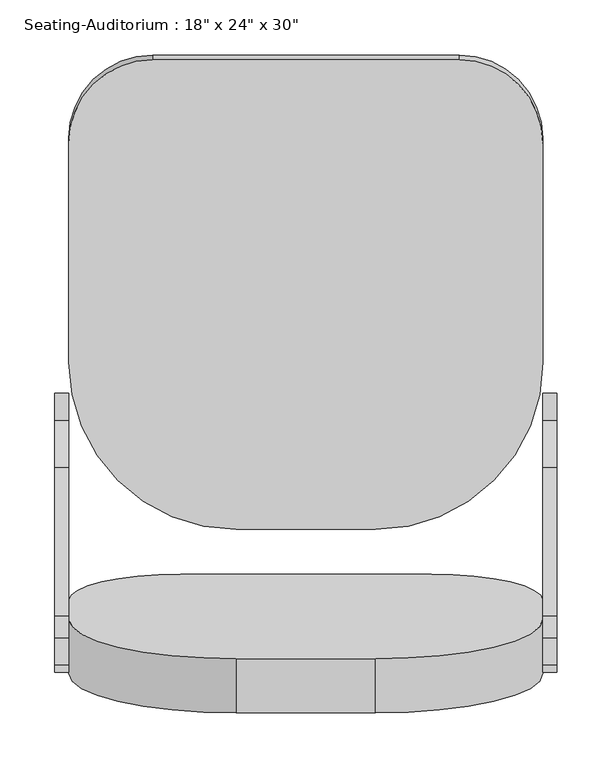
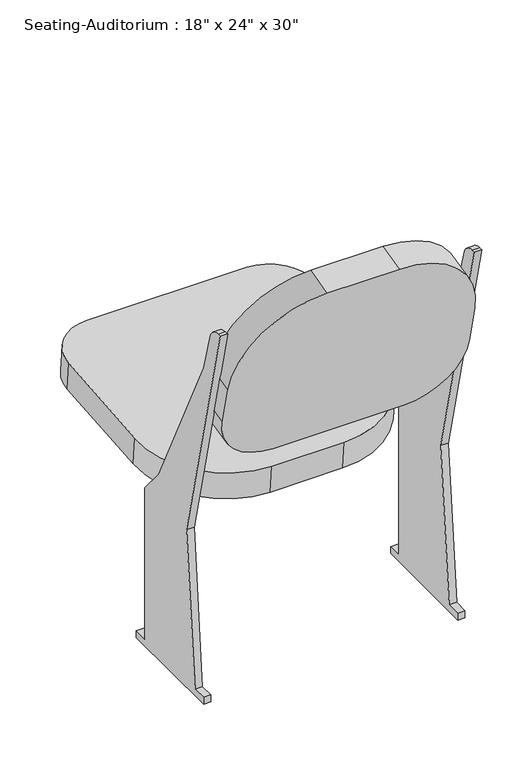
"""IFC4 building model written with IfcOpenShell, lengths in millimetres: furniture geometry."""

from ifc_helpers import new_model, si_unit, point, frame, frame_2d, origin, place, context, project, spatial, polyline, circle_curve, trimmed, segment, composite_curve, outline, extrude, source, transform, mapped, element, save


def furniture_3d1d9cbc(model_context):
    return source(origin(), model_context, "Body", "SweptSolid", [
        extrude(outline(composite_curve([segment(polyline([(0.0, 0.0), (127.0, 0.0)]), True, "CONTINUOUS"), segment(trimmed(circle_curve(frame_2d((127.0, -152.4)), 152.4), [point((127.0, 0.0))], [point((279.4, -152.4))], False, "CARTESIAN"), True, "CONTINUOUS"), segment(polyline([(279.4, -152.4), (279.4, -224.0588601)]), True, "CONTINUOUS"), segment(trimmed(circle_curve(frame_2d((177.8, -224.0588601)), 101.6), [point((279.4, -224.0588601))], [point((177.8, -325.6588601))], False, "CARTESIAN"), True, "CONTINUOUS"), segment(polyline([(177.8, -325.6588601), (-50.8, -325.6588601)]), True, "CONTINUOUS"), segment(trimmed(circle_curve(frame_2d((-50.8, -224.0588601)), 101.6), [point((-50.8, -325.6588601))], [point((-152.4, -224.0588601))], False, "CARTESIAN"), True, "CONTINUOUS"), segment(polyline([(-152.4, -224.0588601), (-152.4, -152.4)]), True, "CONTINUOUS"), segment(trimmed(circle_curve(frame_2d((0.0, -152.4)), 152.4), [point((-152.4, -152.4))], [point((0.0, 0.0))], False, "CARTESIAN"), True, "CONTINUOUS")], self_intersect=False)), frame((224.2278689, -101.3396919, 755.9484479), z_axis=(0.0, 0.9717404775047361, 0.23605178325712217), x_axis=(-1.0, 0.0, 0.0)), (0.0, 0.0, 1.0), 50.8),
        extrude(outline(composite_curve([segment(trimmed(circle_curve(frame_2d((0.0, -76.2)), 76.2), [point((0.0, 0.0))], [point((76.2, -76.2))], False, "CARTESIAN"), True, "CONTINUOUS"), segment(polyline([(76.2, -76.2), (76.2, -276.4123505)]), True, "CONTINUOUS"), segment(trimmed(circle_curve(frame_2d((-76.2, -276.4123505)), 152.4), [point((76.2, -276.4123505))], [point((-76.2, -428.8123506))], False, "CARTESIAN"), True, "CONTINUOUS"), segment(polyline([(-76.2, -428.8123506), (-203.2, -428.8123506)]), True, "CONTINUOUS"), segment(trimmed(circle_curve(frame_2d((-203.2, -276.4123505)), 152.4), [point((-203.2, -428.8123506))], [point((-355.6, -276.4123505))], False, "CARTESIAN"), True, "CONTINUOUS"), segment(polyline([(-355.6, -276.4123505), (-355.6, -76.2)]), True, "CONTINUOUS"), segment(trimmed(circle_curve(frame_2d((-279.4, -76.2)), 76.2), [point((-355.6, -76.2))], [point((-279.4, 0.0))], False, "CARTESIAN"), True, "CONTINUOUS"), segment(polyline([(-279.4, 0.0), (0.0, 0.0)]), True, "CONTINUOUS")], self_intersect=False)), frame((300.4278689, 497.5245173, 321.2380213), z_axis=(0.0, -0.08715574274765496, 0.9961946980917459), x_axis=(1.0, 0.0, 0.0)), (0.0, 0.0, 1.0), 50.8),
        extrude(outline(composite_curve([segment(polyline([(-13.3245902, 0.0), (-13.3245902, 12.7), (12.0754098, 12.7), (37.4754098, 292.1), (-64.1245902, 711.2), (-57.883846, 711.2)]), True, "CONTINUOUS"), segment(trimmed(circle_curve(frame_2d((-57.883846, 685.8)), 25.4), [point((-57.883846, 711.2))], [point((-33.4611378, 692.7779166))], False, "CARTESIAN"), True, "CONTINUOUS"), segment(polyline([(-33.4611378, 692.7779166), (-13.3245902, 622.3), (121.8491486, 342.9), (164.4754098, 292.1), (164.4754098, 12.7), (189.8754098, 12.7), (189.8754098, 0.0), (-13.3245902, 0.0)]), True, "CONTINUOUS")], self_intersect=False)), frame((-67.8721311, 0.0, 0.0), z_axis=(1.0, 0.0, 0.0), x_axis=(0.0, 1.0, 0.0)), (0.0, 0.0, 1.0), 12.7),
        extrude(outline(composite_curve([segment(polyline([(-13.3245902, 12.7), (12.0754098, 12.7), (37.4754098, 292.1), (-64.1245902, 711.2), (-57.883846, 711.2)]), True, "CONTINUOUS"), segment(trimmed(circle_curve(frame_2d((-57.883846, 685.8)), 25.4), [point((-57.883846, 711.2))], [point((-33.4611378, 692.7779166))], False, "CARTESIAN"), True, "CONTINUOUS"), segment(polyline([(-33.4611378, 692.7779166), (-13.3245902, 622.3), (121.8491486, 342.9), (164.4754098, 292.1), (164.4754098, 12.7), (189.8754098, 12.7), (189.8754098, 0.0), (-13.3245902, 0.0), (-13.3245902, 12.7)]), True, "CONTINUOUS")], self_intersect=False)), frame((376.6278689, 0.0, 0.0), z_axis=(1.0, 0.0, 0.0), x_axis=(0.0, 1.0, 0.0)), (0.0, 0.0, 1.0), 12.7),
    ])


if __name__ == "__main__":
    model = new_model("IFC4")
    model_context = context("Model", 3, world=origin())
    ifc_project = project(units=[si_unit("LENGTHUNIT", "METRE", prefix="MILLI")], contexts=[model_context])
    site = spatial("IfcSite", under=ifc_project)
    building = spatial("IfcBuilding", under=site)
    placement = place(None, origin())
    furniture_shape = furniture_3d1d9cbc(model_context)
    element("IfcFurniture", 1, ObjectType="Seating-Auditorium : 18\" x 24\" x 30\"", at=placement, inside=building, context=model_context, shape_type="MappedRepresentation", body=[
        mapped(furniture_shape, transform((0.0, 0.0, 0.0), x_axis=(1.0, 0.0, 0.0), y_axis=(0.0, 1.0, 0.0), z_axis=(0.0, 0.0, 1.0))),
    ])
    save(model, "model.ifc")

# Revit data of these elements
# Type "Seating-Auditorium : 18\" x 24\" x 30\""
#   Assembly Code = "E2020200"
#   Seat Material = Linen, Beige
#   Frame Material = Steel, Paint Finish, Dark Gray, Matte
#   Default Elevation = 0
# Element 1 (IfcFurniture, "Seating-Auditorium : 18\" x 24\" x 30\"")
#   Materials on its faces: "Steel, Paint Finish, Dark Gray, Matte", "Linen, Beige"
# Materials
#   "Linen, Beige": class "Textile", colour RGB 249 239 230, transparency 0, Description = "Linen, beige", Cost = 0
#   "Steel, Paint Finish, Dark Gray, Matte": class "Metal", colour RGB 98 98 98, transparency 0, Description = "Steel, paint finish, dark gray, matte", Cost = 0
